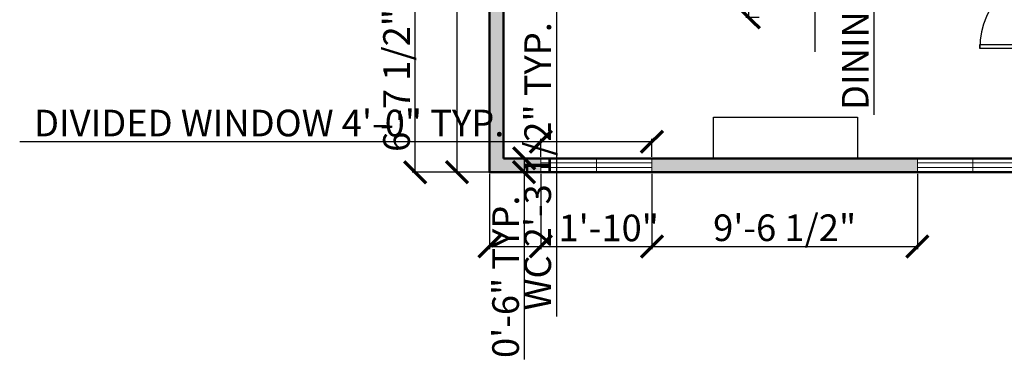
# Model space of a CAD drawing. Units: inches. Extents: x 3147 to 3847, y 1414 to 2207.
# Tile 1 of 7: x 3147 to 3572, y 1414 to 1561. Entities that reach past the tile are written whole.
import ezdxf

# ---------------------------------------------------------------- set-up
doc = ezdxf.new("R2010")
doc.units = ezdxf.units.IN
for name, color, linetype, lineweight in [('A-ANNO-DIMS', 2, 'Continuous', 18), ('A-DOOR', 3, 'Continuous', 25), ('A-FLOR-CASE', 32, 'Continuous', 25), ('A-GLAZ', 4, 'Continuous', 18), ('A-WALL', 7, 'Continuous', 50)]:
    doc.layers.add(name, color=color, linetype=linetype, lineweight=lineweight)
doc.layers.add('A-WALL-PATT', color=18, linetype='Continuous', lineweight=13, true_color=0x000000)
doc.styles.get("Standard").update_dxf_attribs({"font": 'arial.ttf'})
doc.dimstyles.new('ISO-25', dxfattribs={"dimtxt": 11.5, "dimasz": 9.5, "dimexe": 1.25, "dimexo": 0.625, "dimtad": 1, "dimdec": 0, "dimlunit": 3, "dimtxsty": 'Standard', "dimblk": 'ARCHTICK', "dimcen": 2.5, "dimadec": 0, "dimazin": 0, "dimtfac": 1, "dimtdec": 0, "dimtmove": 0, "dimatfit": 3, "dimfxl": 1, "dimarcsym": 0})

# ---------------------------------------------------------------- blocks, each defined once
blk = doc.blocks.new('*U6')
for p, q in [((0, 0), (0, -100)), ((900, 0), (900, -100))]:
    blk.add_line(p, q)
blk.add_lwpolyline([(0, 0), (0, 900), (43.75, 900), (43.75, 0)], close=True)
blk.add_arc((0, 0), 900, 0, 90)
blk = doc.blocks.new('_ArchTick')
at = {"color": 0, "linetype": 'ByBlock', "const_width": 0.15}
blk.add_lwpolyline([(-0.5, -0.5), (0.5, 0.5)], dxfattribs=at)
blk = doc.blocks.new('*D22')
at = {"layer": 'A-ANNO-DIMS', "color": 0, "lineweight": -2, "transparency": 16777216}
for p, q in [((3349.14, 2093.05), (3334.5, 2093.05)), ((3335.75, 2093.05), (3335.75, 1495.05)), ((3349.14, 1495.05), (3334.5, 1495.05))]:
    blk.add_line(p, q, dxfattribs=at)
at = {"layer": 'Defpoints', "color": 0, "transparency": 16777216}
for p in [(3349.76, 2093.05), (3335.75, 1495.05), (3349.76, 1495.05)]:
    blk.add_point(p, dxfattribs=at)
at = {"layer": 'A-ANNO-DIMS', "color": 0, "lineweight": -2, "transparency": 16777216, "xscale": 9.5, "yscale": 9.5, "zscale": 9.5}
for p, rotation in [((3335.75, 2093.05), 90), ((3335.75, 1495.05), 270)]:
    blk.add_blockref('_ArchTick', p, dxfattribs=dict(at, rotation=rotation))
at = {"layer": 'A-ANNO-DIMS', "color": 0, "transparency": 16777216, "insert": (3329.25, 1794.05), "char_height": 11.5, "attachment_point": 5, "rotation": 90}
blk.add_mtext('49\'-10"', dxfattribs=at)
blk = doc.blocks.new('WIN-48IN-DIVIDED')
for p, q in [((0, 6), (0, 0)), ((24, 6), (24, 0)), ((48, 6), (48, 0)), ((48, 4), (0, 4))]:
    blk.add_line(p, q)
blk.add_lwpolyline([(48, 2), (0, 2)])
blk = doc.blocks.new('*D31')
at = {"layer": 'A-ANNO-DIMS', "color": 0, "lineweight": -2, "transparency": 16777216}
for p, q in [((3382.17, 1599.72), (3377.4, 1599.72)), ((3378.65, 1599.72), (3378.65, 1572.05)), ((3382.17, 1572.05), (3377.4, 1572.05)), ((3378.65, 1572.05), (3378.65, 1432.7))]:
    blk.add_line(p, q, dxfattribs=at)
at = {"layer": 'Defpoints', "color": 0, "transparency": 16777216}
for p in [(3382.8, 1599.72), (3378.65, 1572.05), (3382.8, 1572.05)]:
    blk.add_point(p, dxfattribs=at)
at = {"layer": 'A-ANNO-DIMS', "color": 0, "lineweight": -2, "transparency": 16777216, "xscale": 9.5, "yscale": 9.5, "zscale": 9.5}
for p, rotation in [((3378.65, 1599.72), 90), ((3378.65, 1572.05), 270)]:
    blk.add_blockref('_ArchTick', p, dxfattribs=dict(at, rotation=rotation))
at = {"layer": 'A-ANNO-DIMS', "color": 0, "transparency": 16777216, "insert": (3372.07, 1497.63), "char_height": 11.5, "attachment_point": 5, "rotation": 90}
blk.add_mtext('WC 2\'-3 1/2" TYP.', dxfattribs=at)
blk = doc.blocks.new('*D39')
at = {"layer": 'A-ANNO-DIMS', "color": 0, "lineweight": -2, "transparency": 16777216}
for p, q in [((3371.89, 1501.67), (3371.89, 1509.5)), ((3419.89, 1501.67), (3419.89, 1509.5)), ((3371.89, 1508.25), (3147.04, 1508.25)), ((3419.89, 1508.25), (3371.89, 1508.25))]:
    blk.add_line(p, q, dxfattribs=at)
at = {"layer": 'Defpoints', "color": 0, "transparency": 16777216}
for p in [(3371.89, 1508.25), (3371.89, 1501.05), (3419.89, 1501.05)]:
    blk.add_point(p, dxfattribs=at)
at = {"layer": 'A-ANNO-DIMS', "color": 0, "lineweight": -2, "transparency": 16777216, "xscale": 9.5, "yscale": 9.5, "zscale": 9.5, "rotation": 180}
blk.add_blockref('_ArchTick', (3371.89, 1508.25), dxfattribs=at)
at = {"layer": 'A-ANNO-DIMS', "color": 0, "lineweight": -2, "transparency": 16777216, "xscale": 9.5, "yscale": 9.5, "zscale": 9.5}
blk.add_blockref('_ArchTick', (3419.89, 1508.25), dxfattribs=at)
at = {"layer": 'A-ANNO-DIMS', "color": 0, "transparency": 16777216, "insert": (3254.72, 1514.82), "char_height": 11.5, "attachment_point": 5}
blk.add_mtext('DIVIDED WINDOW 4\'-0" TYP.', dxfattribs=at)
blk = doc.blocks.new('*D40')
at = {"layer": 'A-ANNO-DIMS', "color": 0, "lineweight": -2, "transparency": 16777216}
for p, q in [((3371.27, 1501.05), (3363.44, 1501.05)), ((3364.69, 1501.05), (3364.69, 1495.05)), ((3371.27, 1495.05), (3363.44, 1495.05)), ((3364.69, 1495.05), (3364.69, 1414.2))]:
    blk.add_line(p, q, dxfattribs=at)
at = {"layer": 'Defpoints', "color": 0, "transparency": 16777216}
for p in [(3371.89, 1501.05), (3364.69, 1495.05), (3371.89, 1495.05)]:
    blk.add_point(p, dxfattribs=at)
at = {"layer": 'A-ANNO-DIMS', "color": 0, "lineweight": -2, "transparency": 16777216, "xscale": 9.5, "yscale": 9.5, "zscale": 9.5}
for p, rotation in [((3364.69, 1501.05), 90), ((3364.69, 1495.05), 270)]:
    blk.add_blockref('_ArchTick', p, dxfattribs=dict(at, rotation=rotation))
at = {"layer": 'A-ANNO-DIMS', "color": 0, "transparency": 16777216, "insert": (3358.2, 1449.88), "char_height": 11.5, "attachment_point": 5, "rotation": 90}
blk.add_mtext('0\'-6" TYP.', dxfattribs=at)
blk = doc.blocks.new('*D43')
at = {"layer": 'A-ANNO-DIMS', "color": 0, "lineweight": -2, "transparency": 16777216}
for p, q in [((3461.63, 1596.11), (3461.63, 1702.01)), ((3466.13, 1596.11), (3460.38, 1596.11)), ((3461.63, 1561.97), (3461.63, 1596.11)), ((3466.13, 1561.97), (3460.38, 1561.97))]:
    blk.add_line(p, q, dxfattribs=at)
at = {"layer": 'Defpoints', "color": 0, "transparency": 16777216}
for p in [(3461.63, 1596.11), (3466.75, 1596.11), (3466.75, 1561.97)]:
    blk.add_point(p, dxfattribs=at)
at = {"layer": 'A-ANNO-DIMS', "color": 0, "lineweight": -2, "transparency": 16777216, "xscale": 9.5, "yscale": 9.5, "zscale": 9.5}
for p, rotation in [((3461.63, 1596.11), 90), ((3461.63, 1561.97), 270)]:
    blk.add_blockref('_ArchTick', p, dxfattribs=dict(at, rotation=rotation))
at = {"layer": 'A-ANNO-DIMS', "color": 0, "transparency": 16777216, "insert": (3455.13, 1653.81), "char_height": 11.5, "attachment_point": 5, "rotation": 90}
blk.add_mtext('TABLE 2\'-10"', dxfattribs=at)
blk = doc.blocks.new('*D49')
at = {"layer": 'A-ANNO-DIMS', "color": 0, "lineweight": -2, "transparency": 16777216}
for p, q in [((3524.58, 1747.43), (3514.41, 1747.43)), ((3515.66, 1747.43), (3515.66, 1683.78)), ((3524.58, 1683.78), (3514.41, 1683.78)), ((3515.66, 1683.78), (3515.66, 1519.84))]:
    blk.add_line(p, q, dxfattribs=at)
at = {"layer": 'Defpoints', "color": 0, "transparency": 16777216}
for p in [(3525.21, 1747.43), (3515.66, 1683.78), (3525.21, 1683.78)]:
    blk.add_point(p, dxfattribs=at)
at = {"layer": 'A-ANNO-DIMS', "color": 0, "lineweight": -2, "transparency": 16777216, "xscale": 9.5, "yscale": 9.5, "zscale": 9.5}
for p, rotation in [((3515.66, 1747.43), 90), ((3515.66, 1683.78), 270)]:
    blk.add_blockref('_ArchTick', p, dxfattribs=dict(at, rotation=rotation))
at = {"layer": 'A-ANNO-DIMS', "color": 0, "transparency": 16777216, "insert": (3509.09, 1597.06), "char_height": 11.5, "attachment_point": 5, "rotation": 90}
blk.add_mtext('DINING SET 5\'-3 1/2"', dxfattribs=at)
blk = doc.blocks.new('*D69')
at = {"layer": 'A-ANNO-DIMS', "color": 0, "lineweight": -2, "transparency": 16777216}
for p, q in [((3349.76, 1494.42), (3349.76, 1461.75)), ((3371.89, 1494.42), (3371.89, 1461.75)), ((3349.76, 1463), (3371.89, 1463)), ((3371.89, 1463), (3421.07, 1463))]:
    blk.add_line(p, q, dxfattribs=at)
at = {"layer": 'Defpoints', "color": 0, "transparency": 16777216}
for p in [(3349.76, 1495.05), (3371.89, 1495.05), (3371.89, 1463)]:
    blk.add_point(p, dxfattribs=at)
at = {"layer": 'A-ANNO-DIMS', "color": 0, "lineweight": -2, "transparency": 16777216, "xscale": 9.5, "yscale": 9.5, "zscale": 9.5, "rotation": 180}
blk.add_blockref('_ArchTick', (3349.76, 1463), dxfattribs=at)
at = {"layer": 'A-ANNO-DIMS', "color": 0, "lineweight": -2, "transparency": 16777216, "xscale": 9.5, "yscale": 9.5, "zscale": 9.5}
blk.add_blockref('_ArchTick', (3371.89, 1463), dxfattribs=at)
at = {"layer": 'A-ANNO-DIMS', "color": 0, "transparency": 16777216, "insert": (3401.23, 1469.5), "char_height": 11.5, "attachment_point": 5}
blk.add_mtext('1\'-10"', dxfattribs=at)
blk = doc.blocks.new('*D70')
at = {"layer": 'A-ANNO-DIMS', "color": 0, "lineweight": -2, "transparency": 16777216}
for p, q in [((3419.89, 1494.42), (3419.89, 1461.75)), ((3534.41, 1494.42), (3534.41, 1461.75)), ((3419.89, 1463), (3534.41, 1463))]:
    blk.add_line(p, q, dxfattribs=at)
at = {"layer": 'Defpoints', "color": 0, "transparency": 16777216}
for p in [(3419.89, 1495.05), (3534.41, 1495.05), (3534.41, 1463)]:
    blk.add_point(p, dxfattribs=at)
at = {"layer": 'A-ANNO-DIMS', "color": 0, "lineweight": -2, "transparency": 16777216, "xscale": 9.5, "yscale": 9.5, "zscale": 9.5, "rotation": 180}
blk.add_blockref('_ArchTick', (3419.89, 1463), dxfattribs=at)
at = {"layer": 'A-ANNO-DIMS', "color": 0, "lineweight": -2, "transparency": 16777216, "xscale": 9.5, "yscale": 9.5, "zscale": 9.5}
blk.add_blockref('_ArchTick', (3534.41, 1463), dxfattribs=at)
at = {"layer": 'A-ANNO-DIMS', "color": 0, "transparency": 16777216, "insert": (3477.15, 1469.57), "char_height": 11.5, "attachment_point": 5}
blk.add_mtext('9\'-6 1/2"', dxfattribs=at)
blk = doc.blocks.new('*D75')
at = {"layer": 'A-ANNO-DIMS', "color": 0, "lineweight": -2, "transparency": 16777216}
for p, q in [((3349.14, 1574.35), (3316.46, 1574.35)), ((3317.71, 1495.05), (3317.71, 1574.35)), ((3349.14, 1495.05), (3316.46, 1495.05))]:
    blk.add_line(p, q, dxfattribs=at)
at = {"layer": 'Defpoints', "color": 0, "transparency": 16777216}
for p in [(3317.71, 1574.35), (3349.76, 1574.35), (3349.76, 1495.05)]:
    blk.add_point(p, dxfattribs=at)
at = {"layer": 'A-ANNO-DIMS', "color": 0, "lineweight": -2, "transparency": 16777216, "xscale": 9.5, "yscale": 9.5, "zscale": 9.5}
for p, rotation in [((3317.71, 1574.35), 90), ((3317.71, 1495.05), 270)]:
    blk.add_blockref('_ArchTick', p, dxfattribs=dict(at, rotation=rotation))
at = {"layer": 'A-ANNO-DIMS', "color": 0, "transparency": 16777216, "insert": (3311.14, 1534.7), "char_height": 11.5, "attachment_point": 5, "rotation": 90}
blk.add_mtext('6\'-7 1/2"', dxfattribs=at)
blk = doc.blocks.new('*D95')
at = {"layer": 'A-ANNO-DIMS', "color": 0, "lineweight": -2, "transparency": 16777216}
for p in [(3490.35, 1721.27), (3490.35, 1547.02)]:
    blk.add_line(p, (3490.35, 1632.65), dxfattribs=at)
at = {"layer": 'Defpoints', "color": 0, "transparency": 16777216}
for p in [(3490.35, 1632.65), (3490.35, 1547.02)]:
    blk.add_point(p, dxfattribs=at)
at = {"layer": 'A-ANNO-DIMS', "color": 0, "lineweight": -2, "transparency": 16777216, "xscale": 9.5, "yscale": 9.5, "zscale": 9.5, "rotation": 270}
blk.add_blockref('_ArchTick', (3490.35, 1632.65), dxfattribs=at)
at = {"layer": 'A-ANNO-DIMS', "color": 0, "transparency": 16777216, "insert": (3483.78, 1686.46), "char_height": 11.5, "attachment_point": 5, "rotation": 90}
blk.add_mtext('R7\'-1 1/2"', dxfattribs=at)
blk = doc.blocks.new('*D96')
at = {"layer": 'A-ANNO-DIMS', "color": 0, "lineweight": -2, "transparency": 16777216}
for p in [(3490.35, 1725.51), (3490.35, 1556.16)]:
    blk.add_line(p, (3490.35, 1636.89), dxfattribs=at)
at = {"layer": 'Defpoints', "color": 0, "transparency": 16777216}
for p in [(3490.35, 1636.89), (3490.35, 1556.16)]:
    blk.add_point(p, dxfattribs=at)
at = {"layer": 'A-ANNO-DIMS', "color": 0, "lineweight": -2, "transparency": 16777216, "xscale": 9.5, "yscale": 9.5, "zscale": 9.5, "rotation": 270}
blk.add_blockref('_ArchTick', (3490.35, 1636.89), dxfattribs=at)
at = {"layer": 'A-ANNO-DIMS', "color": 0, "transparency": 16777216, "insert": (3483.78, 1690.7), "char_height": 11.5, "attachment_point": 5, "rotation": 90}
blk.add_mtext('R6\'-8 1/2"', dxfattribs=at)

msp = doc.modelspace()

# ---------------------------------------------------------------- hatches: boundary and pattern name
at = {"layer": 'A-WALL-PATT'}
h = msp.add_hatch(color=256, dxfattribs=at)
h.dxf.hatch_style = 1
h.paths.add_polyline_path([(3616.76, 2093.05), (3594.02, 2093.05), (3594.02, 2087.05), (3611.76, 2087.05), (3611.76, 1993.05), (3616.76, 1993.05), (3628.76, 1993.05), (3628.76, 1996.99), (3628.76, 1998.05), (3616.76, 1998.05), (3616.76, 2087.05)])
h.paths.add_polyline_path([(3576.44, 2093.05), (3527.03, 2093.05), (3527.03, 2087.05), (3546.76, 2087.05), (3546.76, 1962.05), (3551.76, 1962.05), (3590.76, 1962.05), (3590.76, 1921.05), (3585.76, 1921.05), (3585.76, 1916.05), (3590.76, 1916.05), (3590.76, 1895.05), (3595.76, 1895.05), (3595.76, 1962.05), (3611.76, 1962.05), (3616.76, 1962.05), (3616.76, 1969.05), (3611.76, 1969.05), (3611.76, 1967.05), (3551.76, 1967.05), (3551.76, 2087.05), (3576.44, 2087.05)])
h.paths.add_polyline_path([(3455.03, 2093.05), (3408.76, 2093.05), (3408.76, 2087.05), (3408.76, 2046.06), (3413.76, 2046.06), (3413.76, 2087.05), (3455.03, 2087.05)])
h.paths.add_polyline_path([(3355.76, 2008.05), (3408.76, 2008.05), (3408.76, 2004.83), (3413.76, 2004.83), (3413.76, 2008.05), (3413.76, 2013.05), (3413.76, 2016.06), (3408.76, 2016.06), (3408.76, 2013.05), (3355.76, 2013.05), (3349.76, 2013.05), (3349.76, 1973.71), (3355.76, 1973.71)])
h.paths.add_polyline_path([(3413.76, 1974.83), (3408.76, 1974.83), (3408.76, 1943.05), (3355.76, 1943.05), (3355.76, 1949.71), (3349.76, 1949.71), (3349.76, 1897.34), (3355.76, 1897.34), (3355.76, 1938.05), (3408.76, 1938.05), (3408.76, 1934.63), (3413.76, 1934.63), (3413.76, 1938.05), (3505.76, 1938.05), (3505.76, 1916.05), (3533.76, 1916.05), (3533.76, 1904.63), (3533.76, 1831.83), (3538.76, 1831.83), (3538.76, 1904.63), (3538.76, 1916.05), (3546.76, 1916.05), (3549.76, 1916.05), (3549.76, 1921.05), (3546.76, 1921.05), (3510.76, 1921.05), (3510.76, 1938.05), (3510.76, 1943.05), (3413.76, 1943.05)])
h.paths.add_polyline_path([(3413.76, 1904.63), (3408.76, 1904.63), (3408.76, 1870.05), (3355.76, 1870.05), (3355.76, 1873.34), (3349.76, 1873.34), (3349.76, 1865.05), (3355.76, 1865.05), (3408.76, 1865.05), (3408.76, 1863.11), (3409.83, 1863.11), (3413.76, 1863.11)], flags=17)
h.paths.add_polyline_path([(3538.76, 1795.83), (3533.76, 1795.83), (3533.76, 1794.05), (3413.76, 1794.05), (3413.76, 1833.11), (3408.76, 1833.11), (3408.76, 1794.05), (3355.76, 1794.05), (3349.76, 1794.05), (3349.76, 1776.88), (3355.76, 1776.88), (3355.76, 1789.05), (3413.76, 1789.05), (3475.76, 1789.05), (3475.76, 1731.91), (3480.76, 1731.91), (3480.76, 1789.05), (3538.76, 1789.05)])
h.paths.add_polyline_path([(3432.14, 1733.05), (3413.76, 1733.05), (3355.76, 1733.05), (3355.76, 1740.88), (3349.76, 1740.88), (3349.76, 1720.47), (3355.76, 1720.47), (3355.76, 1729.05), (3413.76, 1729.05), (3432.14, 1729.05)])
h.paths.add_polyline_path([(3480.76, 1695.91), (3476.83, 1695.91), (3475.76, 1695.91), (3475.76, 1693.05), (3413.76, 1693.05), (3355.76, 1693.05), (3355.76, 1696.47), (3349.76, 1696.47), (3349.76, 1671.27), (3355.76, 1671.27), (3355.76, 1688.05), (3413.76, 1688.05), (3415.76, 1688.05), (3415.76, 1673.71), (3420.76, 1673.71), (3420.76, 1688.05), (3480.76, 1688.05)])
h.paths.add_polyline_path([(3420.76, 1643.71), (3415.76, 1643.71), (3415.76, 1642.05), (3413.76, 1642.05), (3355.76, 1642.05), (3355.76, 1647.27), (3349.76, 1647.27), (3349.76, 1598.35), (3355.76, 1598.35), (3355.76, 1637.05), (3401.76, 1637.05), (3401.76, 1634.26), (3406.76, 1634.26), (3406.76, 1637.05), (3413.76, 1637.05), (3420.76, 1637.05)])
h.paths.add_polyline_path([(3406.76, 1604.26), (3401.76, 1604.26), (3401.76, 1572.05), (3355.76, 1572.05), (3355.76, 1574.35), (3349.76, 1574.35), (3349.76, 1553.05), (3349.76, 1495.05), (3371.89, 1495.05), (3371.89, 1501.05), (3355.76, 1501.05), (3355.76, 1559.05), (3355.76, 1567.05), (3406.76, 1567.05), (3406.76, 1572.05)])
h.paths.add_polyline_path([(3534.41, 1501.05), (3419.89, 1501.05), (3419.89, 1495.05), (3534.41, 1495.05)])
h.paths.add_polyline_path([(3769.76, 1509.48), (3763.76, 1509.48), (3763.76, 1501.05), (3600.76, 1501.05), (3600.76, 1548.51), (3595.76, 1548.51), (3595.76, 1501.05), (3582.41, 1501.05), (3582.41, 1495.05), (3769.76, 1495.05)])
h.paths.add_polyline_path([(3769.76, 1645.82), (3763.76, 1645.82), (3763.76, 1593.05), (3664.76, 1593.05), (3619.76, 1593.05), (3619.76, 1674.05), (3614.76, 1674.05), (3614.76, 1593.05), (3595.76, 1593.05), (3595.76, 1584.51), (3600.76, 1584.51), (3600.76, 1588.05), (3619.76, 1588.05), (3664.76, 1588.05), (3763.76, 1588.05), (3763.76, 1569.48), (3769.76, 1569.48)])
h.paths.add_polyline_path([(3769.76, 1731.24), (3763.76, 1731.24), (3763.76, 1718.05), (3664.76, 1718.05), (3595.76, 1718.05), (3595.76, 1723.05), (3590.76, 1723.05), (3590.76, 1713.05), (3595.76, 1713.05), (3614.76, 1713.05), (3614.76, 1710.05), (3619.76, 1710.05), (3619.76, 1713.05), (3664.76, 1713.05), (3763.76, 1713.05), (3763.76, 1693.82), (3769.76, 1693.82)])
h.paths.add_polyline_path([(3769.76, 1872.64), (3763.76, 1872.64), (3763.76, 1854.05), (3664.76, 1854.05), (3595.76, 1854.05), (3595.76, 1859.05), (3590.76, 1859.05), (3590.76, 1759.05), (3595.76, 1759.05), (3595.76, 1849.05), (3664.76, 1849.05), (3763.76, 1849.05), (3763.76, 1815.24), (3769.76, 1815.24)])
h.paths.add_polyline_path([(3769.76, 1998.05), (3763.76, 1998.05), (3763.76, 1968.64), (3769.76, 1968.64)])
h.paths.add_polyline_path([(3763.76, 1998.05), (3664.76, 1998.05), (3664.76, 1993.05), (3763.76, 1993.05)])

# ---------------------------------------------------------------- linework, layer by layer
at = {"layer": 'A-FLOR-CASE'}
for p, q in [((3446.47, 1501.05), (3446.47, 1518.88)), ((3446.47, 1518.88), (3508.63, 1518.88)), ((3508.63, 1518.88), (3508.63, 1501.05))]:
    msp.add_line(p, q, dxfattribs=at)
at = {"layer": 'A-WALL'}
for p, q in [((3349.76, 1553.05), (3349.76, 2093.05)), ((3355.76, 1559.05), (3355.76, 1567.05)), ((3355.76, 1501.05), (3355.76, 1559.05)), ((3595.76, 1501.05), (3355.76, 1501.05))]:
    msp.add_line(p, q, dxfattribs=at)
msp.add_lwpolyline([(3769.76, 1553.05), (3769.76, 1495.05), (3349.76, 1495.05), (3349.76, 1553.05)], dxfattribs=at)

# ---------------------------------------------------------------- block references
at = {"layer": 'A-DOOR', "xscale": 0.0393700787401575, "yscale": 0.0393700787401575, "zscale": 0.0393700787401575, "rotation": 89.99999999999999}
msp.add_blockref('*U6', (3596.83, 1548.51), dxfattribs=at)
at = {"layer": 'A-GLAZ', "rotation": 180}
msp.add_blockref('WIN-48IN-DIVIDED', (3419.89, 1501.05), dxfattribs=at)
at = {"layer": 'A-GLAZ'}
msp.add_blockref('WIN-48IN-DIVIDED', (3534.41, 1495.05), dxfattribs=at)

# ---------------------------------------------------------------- dimensions: what is measured, and where the dimension line sits
at = {"layer": 'A-ANNO-DIMS'}
for base, p1, p2, override, picture, middle in [((3335.75, 1495.05), (3349.76, 2093.05), (3349.76, 1495.05), {"dimclrd": 0, "dimclre": 0, "dimclrt": 0}, '*D22', (3329.25, 1794.05)), ((3317.71, 1574.35), (3349.76, 1495.05), (3349.76, 1574.35), {"dimdec": 1, "dimlfac": 1, "dimrnd": 0, "dimzin": 1, "dimdsep": 46, "dimlunit": 4, "dimfrac": 2}, '*D75', (3311.14, 1534.7))]:
    dim = msp.add_linear_dim(base=base, p1=p1, p2=p2, angle=90, dimstyle='ISO-25', override=override, dxfattribs=at)
    dim.commit()
    dim.dimension.update_dxf_attribs({"geometry": picture, "text_midpoint": middle})
for base, p1, p2, angle, text, picture, middle in [((3515.6604, 1683.7807), (3525.2085, 1747.4344), (3525.2085, 1683.7807), 270, 'DINING SET <>', '*D49', (3509.0854, 1597.0583)), ((3461.63, 1596.11), (3466.75, 1561.97), (3466.75, 1596.11), 90, 'TABLE <>', '*D43', (3455.13, 1653.81)), ((3378.65, 1572.05), (3382.8, 1599.72), (3382.8, 1572.05), 270, 'WC <> TYP.', '*D31', (3372.07, 1497.63)), ((3371.89, 1508.25), (3419.89, 1501.05), (3371.89, 1501.05), 180, 'DIVIDED WINDOW <> TYP.', '*D39', (3254.72, 1514.82)), ((3364.69, 1495.05), (3371.89, 1501.05), (3371.89, 1495.05), 270, '<> TYP.', '*D40', (3358.2, 1449.88))]:
    dim = msp.add_linear_dim(base=base, p1=p1, p2=p2, angle=angle, text=text, dimstyle='ISO-25', override={"dimdec": 1, "dimlfac": 1, "dimrnd": 0, "dimzin": 1, "dimdsep": 46, "dimlunit": 4, "dimfrac": 2}, dxfattribs=at)
    dim.commit()
    dim.dimension.update_dxf_attribs({"geometry": picture, "text_midpoint": middle})
for center, mpoint, picture, middle in [((3490.35, 1556.16), (3490.35, 1636.89), '*D96', (3483.78, 1690.7)), ((3490.35, 1547.02), (3490.35, 1632.65), '*D95', (3483.78, 1686.46))]:
    dim = msp.add_radius_dim(center=center, mpoint=mpoint, dimstyle='ISO-25', override={"dimdec": 1, "dimlfac": 1, "dimrnd": 0, "dimzin": 1, "dimdsep": 46, "dimlunit": 4, "dimfrac": 2}, dxfattribs=at)
    dim.commit()
    dim.dimension.update_dxf_attribs({"geometry": picture, "text_midpoint": middle})
for base, p1, p2, picture, middle in [((3371.89, 1463), (3349.76, 1495.05), (3371.89, 1495.05), '*D69', (3401.23, 1469.5)), ((3534.41, 1463), (3419.89, 1495.05), (3534.41, 1495.05), '*D70', (3477.15, 1469.57))]:
    dim = msp.add_linear_dim(base=base, p1=p1, p2=p2, dimstyle='ISO-25', override={"dimdec": 1, "dimlfac": 1, "dimrnd": 0, "dimzin": 1, "dimdsep": 46, "dimlunit": 4, "dimfrac": 2}, dxfattribs=at)
    dim.commit()
    dim.dimension.update_dxf_attribs({"geometry": picture, "text_midpoint": middle})

doc.saveas('drawing.dxf')
